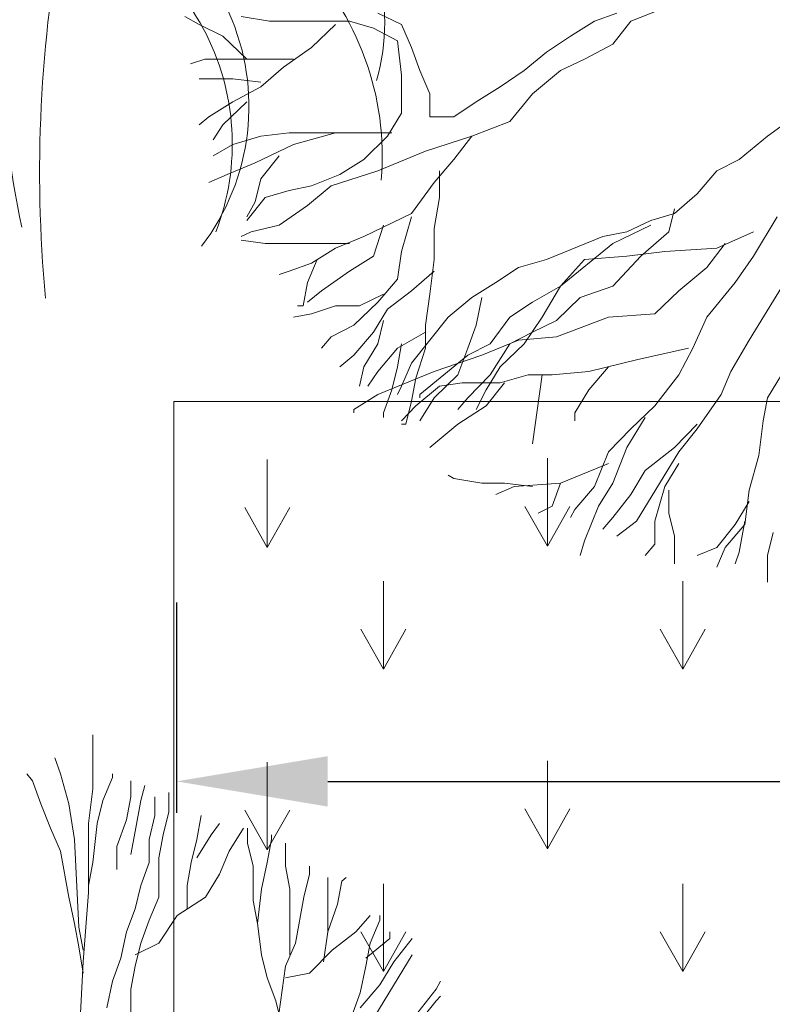
# Model space of a CAD drawing. Units: millimetres. Extents: x 595116 to 630915, y 909473 to 920225.
# Tile 48 of 134: x 629529 to 629559, y 919242 to 919281. Entities that reach past the tile are written whole.
import ezdxf

# ---------------------------------------------------------------- set-up
doc = ezdxf.new("R2010")
doc.units = ezdxf.units.MM
doc.layers.add('Dimension', color=3, linetype='Continuous', lineweight=18)
doc.layers.add('L-PLNT', color=85, linetype='Continuous', lineweight=13)
doc.styles.get("Standard").update_dxf_attribs({"font": 'arial.ttf'})
doc.dimstyles.new('ISO-25', dxfattribs={"dimtxt": 9, "dimasz": 6, "dimexe": 1.25, "dimexo": 0.625, "dimtad": 1, "dimlunit": 4, "dimtxsty": 'Standard', "dimcen": 2.5, "dimadec": 0, "dimazin": 0, "dimtfac": 1, "dimtmove": 0, "dimatfit": 3, "dimfxl": 1, "dimarcsym": 0})

# ---------------------------------------------------------------- blocks, each defined once
blk = doc.blocks.new('tree')
for centre, radius, start, end in [((629595.141, 919296.95), 5.184, 352.032, 57.0714), ((629569.835, 919289.496), 31.168, 13.149, 20.5076), ((629604.232, 919296.737), 3.791, 61.1347, 193.108), ((629594.259, 919292.132), 6.965, 7.4001, 94.0059), ((629589.446, 919288.922), 12.167, 24.2477, 54.3726), ((629605.429, 919293.205), 4.185, 348.9977, 176.315), ((629605.915, 919293.144), 3.963, 69.3845, 175.231), ((629595.377, 919292.044), 4.722, 54.2484, 144.2167), ((629594.88, 919291.171), 5.506, 43.8672, 89.4805), ((629597.025, 919289.989), 5.01, 36.0581, 170.6542), ((629596.464, 919289.874), 4.4, 52.9074, 159.3471), ((629603.809, 919290.469), 3.92, 343.886, 112.2662), ((629598.153, 919288.998), 5.103, 105.3576, 208.8973), ((629597.068, 919289.758), 3.768, 80.4816, 161.0664), ((629601.247, 919287.941), 5.545, 101.0419, 191.8692), ((629614.329, 919289.554), 13.748, 164.5925, 192.323), ((629600.849, 919288.894), 4.324, 322.5461, 85.805), ((629602.329, 919287.957), 5.355, 355.2141, 94.8217), ((629602.391, 919286.088), 6.769, 99.681, 184.5451), ((629600.275, 919288.191), 4.585, 338.7925, 77.6921), ((629626.813, 919287.645), 25.579, 169.0753, 185.2889)]:
    blk.add_arc(centre, radius, start, end)
blk = doc.blocks.new('A$C143125F4')
for p, q in [((2.883, 4.8338), (2.883, 5.0443)), ((2.7571, 4.892), (2.7353, 4.9547)), ((2.6477, 4.8651), (2.6259, 4.892)), ((2.6806, 4.7755), (2.6477, 4.8651)), ((2.79, 4.7755), (2.7571, 4.892)), ((2.9213, 4.789), (2.9596, 4.8786)), ((2.9596, 4.8786), (2.9596, 4.892)), ((3.0307, 4.8024), (3.0307, 4.8651)), ((2.8666, 4.6994), (2.883, 4.8338)), ((3.069, 4.789), (3.0854, 4.8472)), ((2.8994, 4.6994), (2.9213, 4.789)), ((3.0143, 4.7128), (3.0307, 4.8024)), ((3.0471, 4.668), (3.069, 4.789)), ((3.1237, 4.7307), (3.1237, 4.8024)), ((3.1784, 4.7442), (3.1784, 4.8203)), ((2.7189, 4.6814), (2.6806, 4.7755)), ((2.8119, 4.6367), (2.79, 4.7755)), ((2.976, 4.6098), (3.0143, 4.7128)), ((3.1018, 4.6367), (3.1237, 4.7307)), ((3.1565, 4.6546), (3.1784, 4.7442)), ((3.2878, 4.6367), (3.3042, 4.7307)), ((2.7571, 4.5919), (2.7189, 4.6814)), ((2.8666, 4.4306), (2.8666, 4.6994)), ((2.883, 4.5471), (2.8994, 4.6994)), ((3.3425, 4.6546), (3.3753, 4.6994)), ((3.4136, 4.5919), (3.4683, 4.6814)), ((3.4847, 4.6232), (3.4847, 4.6814)), ((2.8283, 4.2962), (2.8119, 4.6367)), ((3.0307, 4.5784), (3.0471, 4.668)), ((3.1018, 4.5471), (3.1018, 4.6367)), ((3.1401, 4.565), (3.1565, 4.6546)), ((3.2659, 4.5471), (3.2878, 4.6367)), ((3.2878, 4.565), (3.3425, 4.6546)), ((3.5613, 4.5471), (3.5777, 4.6367)), ((3.5777, 4.6367), (3.5777, 4.6546)), ((2.976, 4.5202), (2.976, 4.6098)), ((3.5066, 4.5336), (3.4847, 4.6232)), ((3.6324, 4.5336), (3.6324, 4.6232)), ((2.79, 4.4127), (2.7571, 4.5919)), ((3.1401, 4.4127), (3.1401, 4.565)), ((3.3753, 4.5023), (3.4136, 4.5919)), ((2.8666, 4.4575), (2.883, 4.5471)), ((3.069, 4.4575), (3.1018, 4.5471)), ((3.2495, 4.4575), (3.2659, 4.5471)), ((3.5066, 4.3992), (3.5066, 4.5336)), ((3.5394, 4.444), (3.5613, 4.5471)), ((3.6488, 4.444), (3.6324, 4.5336)), ((3.7254, 4.5023), (3.7254, 4.5336)), ((3.3206, 4.4127), (3.3753, 4.5023)), ((3.7035, 4.4127), (3.7254, 4.5023)), ((3.7965, 4.2783), (3.7965, 4.4888)), ((3.8512, 4.4754), (3.8677, 4.4888)), ((3.0471, 4.3679), (3.069, 4.4575)), ((3.2495, 4.3679), (3.2495, 4.4575)), ((3.523, 4.3096), (3.5394, 4.444)), ((3.6488, 4.1887), (3.6488, 4.444)), ((3.8348, 4.3858), (3.8512, 4.4754)), ((2.8119, 4.3096), (2.79, 4.4127)), ((2.8447, 4.1618), (2.8666, 4.4306)), ((3.1018, 4.3231), (3.1401, 4.4127)), ((3.2112, 4.341), (3.3206, 4.4127)), ((3.6707, 4.2335), (3.7035, 4.4127)), ((3.0143, 4.2783), (3.0471, 4.3679)), ((3.523, 4.3096), (3.5066, 4.3992)), ((3.7965, 4.2783), (3.8348, 4.3858)), ((3.1401, 4.2335), (3.2112, 4.341)), ((3.906, 4.2783), (3.9607, 4.341)), ((3.999, 4.3231), (3.999, 4.341)), ((2.8283, 4.22), (2.8119, 4.3096)), ((2.8447, 4.2066), (2.8283, 4.2962)), ((3.069, 4.2335), (3.1018, 4.3231)), ((3.5394, 4.1887), (3.523, 4.3096)), ((3.9607, 4.2335), (3.999, 4.3231)), ((2.9924, 4.1752), (3.0143, 4.2783)), ((3.7801, 4.1618), (3.7965, 4.2783)), ((3.813, 4.2066), (3.906, 4.2783)), ((3.9442, 4.1752), (4.0372, 4.2514)), ((4.0372, 4.2514), (4.0372, 4.2783)), ((4.1248, 4.2514), (4.0537, 4.1618)), ((2.8447, 4.117), (2.8283, 4.22)), ((3.0471, 4.1887), (3.1401, 4.2335)), ((3.0471, 4.1439), (3.069, 4.2335)), ((3.6324, 4.1439), (3.6707, 4.2335)), ((3.9442, 4.1439), (3.9607, 4.2335)), ((2.9596, 4.0856), (2.9924, 4.1752)), ((3.5613, 4.0991), (3.5394, 4.1887)), ((3.7254, 4.117), (3.813, 4.2066)), ((3.9607, 3.9199), (4.1248, 4.1887)), ((2.8283, 3.8303), (2.8447, 4.1618)), ((3.0307, 4.0543), (3.0471, 4.1439)), ((3.5941, 3.8751), (3.6324, 4.1439)), ((3.9224, 4.0408), (3.9442, 4.1439)), ((4.0537, 4.1618), (3.999, 4.0722)), ((3.5941, 4.0095), (3.5613, 4.0991)), ((3.6324, 4.0991), (3.7254, 4.117)), ((2.9377, 3.9826), (2.9596, 4.0856)), ((3.999, 4.0722), (3.9224, 3.9826)), ((4.2178, 4.0543), (4.2342, 4.0856)), ((3.0307, 3.9647), (3.0307, 4.0543)), ((3.8895, 3.9512), (3.9224, 4.0408)), ((4.1467, 3.9647), (4.2178, 4.0543)), ((4.2178, 4.0095), (4.2342, 4.0274)), ((3.616, 3.9199), (3.5941, 4.0095)), ((4.1467, 3.9199), (4.2178, 4.0095)), ((0.7823, 2.231), (0.8753, 2.1862)), ((1.6247, 2.1996), (1.7123, 2.231)), ((1.8819, 2.2444), (1.767, 2.1996)), ((0.0875, 2.1862), (0.0328, 2.2175)), ((0.1805, 2.1414), (0.0875, 2.1862)), ((0.3611, 2.1996), (0.2516, 2.2175)), ((0.6729, 2.1996), (0.3611, 2.1996)), ((0.6182, 2.1862), (0.5252, 2.0966)), ((0.7659, 2.1727), (0.6729, 2.1996)), ((0.8753, 2.1862), (0.9136, 2.0966)), ((1.5317, 2.1414), (1.6247, 2.1996)), ((1.767, 2.1996), (1.6959, 2.11)), ((0.8589, 2.1235), (0.7659, 2.1727)), ((0.2735, 2.0518), (0.1805, 2.1414)), ((0.8753, 1.9891), (0.8589, 2.1235)), ((1.4387, 2.0787), (1.5317, 2.1414)), ((1.6959, 2.11), (1.5865, 2.0518)), ((0.5252, 2.0966), (0.4158, 2.0204)), ((0.9136, 2.0966), (0.9464, 2.007)), ((1.3512, 2.007), (1.4387, 2.0787)), ((0.1094, 2.0518), (0.0547, 2.0339)), ((0.4541, 2.0518), (0.1094, 2.0518)), ((1.5865, 2.0518), (1.4935, 2.007)), ((0.4158, 2.0204), (0.3282, 1.9443)), ((0.9464, 2.007), (0.9847, 1.9174)), ((1.2582, 1.9443), (1.3512, 2.007)), ((1.4935, 2.007), (1.384, 1.9174)), ((0.2188, 1.9756), (0.0875, 1.9756)), ((0.3282, 1.9622), (0.2188, 1.9756)), ((0.8753, 1.8412), (0.8753, 1.9891)), ((0.3282, 1.9443), (0.2188, 1.886)), ((0.9847, 1.9174), (0.9847, 1.8278)), ((1.1652, 1.886), (1.2582, 1.9443)), ((1.384, 1.9174), (1.2965, 1.8099)), ((0.2188, 1.886), (0.1258, 1.8278)), ((0.2735, 1.886), (0.1805, 1.7964)), ((1.0777, 1.8278), (1.1652, 1.886)), ((2.5, 1.8995), (2.2976, 1.7516)), ((0.8206, 1.7516), (0.8753, 1.8412)), ((0.1258, 1.8278), (0.0875, 1.7964)), ((0.9847, 1.8278), (1.0777, 1.8278)), ((1.2965, 1.8099), (1.1488, 1.7516)), ((0.1805, 1.7964), (0.1422, 1.7382)), ((0.4376, 1.7651), (0.3282, 1.7516)), ((0.837, 1.7651), (0.4376, 1.7651)), ((0.6182, 1.7651), (0.4541, 1.7203)), ((0.3282, 1.7516), (0.2188, 1.7203)), ((0.7276, 1.662), (0.8206, 1.7516)), ((1.1488, 1.7516), (0.9683, 1.6934)), ((1.1488, 1.7516), (1.0777, 1.662)), ((2.2976, 1.7516), (2.1882, 1.662)), ((0.2188, 1.7203), (0.1422, 1.6755)), ((0.4541, 1.7203), (0.3063, 1.6486)), ((0.9683, 1.6934), (0.7823, 1.6172)), ((0.3063, 1.6486), (0.1969, 1.6038)), ((0.3993, 1.6755), (0.3282, 1.5859)), ((0.6346, 1.6038), (0.7276, 1.662)), ((1.0777, 1.662), (1.0011, 1.5724)), ((2.1882, 1.662), (2.1007, 1.6172)), ((0.7823, 1.6172), (0.6018, 1.559)), ((1.023, 1.6172), (1.023, 1.5142)), ((2.1007, 1.6172), (2.0241, 1.5276)), ((0.1969, 1.6038), (0.1258, 1.5724)), ((0.3282, 1.5859), (0.3063, 1.4963)), ((0.5252, 1.559), (0.6346, 1.6038)), ((1.0011, 1.5724), (0.9136, 1.4515)), ((0.3446, 1.5142), (0.4376, 1.5411)), ((0.4376, 1.5411), (0.5252, 1.559)), ((0.6018, 1.559), (0.5088, 1.4828)), ((0.2735, 1.4246), (0.3446, 1.5142)), ((0.3063, 1.4963), (0.2735, 1.438)), ((1.023, 1.5142), (1.0011, 1.3932)), ((2.0241, 1.5276), (1.9366, 1.4515)), ((0.5088, 1.4828), (0.3993, 1.4067)), ((1.9366, 1.4694), (1.9147, 1.3798)), ((0.9136, 1.4515), (0.7276, 1.3619)), ((0.9136, 1.438), (0.8753, 1.3036)), ((1.8436, 1.4246), (1.7506, 1.3798)), ((1.9366, 1.4515), (1.8436, 1.4246)), ((2.3359, 1.438), (2.2429, 1.2857)), ((0.2899, 1.3798), (0.2516, 1.3619)), ((0.3993, 1.4067), (0.2899, 1.3798)), ((0.8042, 1.4067), (0.7659, 1.2857)), ((1.0011, 1.3932), (1.0011, 1.2723)), ((1.7506, 1.3798), (1.6576, 1.3619)), ((1.8436, 1.4067), (1.6959, 1.335)), ((1.9147, 1.3798), (1.8053, 1.2857)), ((2.2429, 1.3798), (2.1007, 1.3171)), ((0.3446, 1.335), (0.2516, 1.3484)), ((0.7276, 1.3619), (0.6182, 1.3171)), ((1.6576, 1.3619), (1.4387, 1.2723)), ((0.6729, 1.335), (0.3446, 1.335)), ((0.6182, 1.3171), (0.5252, 1.2588)), ((0.8753, 1.3036), (0.8589, 1.1961)), ((1.6959, 1.335), (1.4935, 1.1692)), ((1.8983, 1.3036), (1.7506, 1.2857)), ((2.1007, 1.3171), (1.8983, 1.3036)), ((2.1335, 1.335), (2.0624, 1.2409)), ((0.5471, 1.2723), (0.5088, 1.1827)), ((0.7659, 1.2857), (0.6729, 1.2275)), ((1.0011, 1.2723), (0.9847, 1.1379)), ((1.4387, 1.2723), (1.3293, 1.2409)), ((1.5865, 1.2723), (1.4935, 1.1692)), ((1.7506, 1.2857), (1.5865, 1.2723)), ((1.8053, 1.2857), (1.6959, 1.1692)), ((2.2429, 1.2857), (2.1718, 1.1827)), ((0.4376, 1.2275), (0.3993, 1.214)), ((0.5252, 1.2588), (0.4376, 1.2275)), ((0.6729, 1.2275), (0.5635, 1.1513)), ((1.0011, 1.2275), (0.9136, 1.1513)), ((1.3293, 1.2409), (1.2418, 1.1827)), ((2.0624, 1.2409), (1.953, 1.1513)), ((2.3906, 1.2275), (2.2265, 0.9587)), ((0.8589, 1.1961), (0.7823, 1.1065)), ((0.5088, 1.1827), (0.4923, 1.0931)), ((0.5635, 1.1513), (0.5088, 1.1065)), ((0.9136, 1.1513), (0.8206, 1.0796)), ((1.2418, 1.1827), (1.1488, 1.1244)), ((1.4935, 1.1692), (1.384, 1.1065)), ((1.4935, 1.1692), (1.4223, 1.0483)), ((1.6959, 1.1692), (1.57, 1.1244)), ((1.953, 1.1513), (1.86, 1.0617)), ((2.1718, 1.1827), (2.0624, 1.0483)), ((0.8042, 1.1379), (0.7112, 1.0931)), ((0.9847, 1.1379), (0.9683, 1.0169)), ((1.1488, 1.1244), (1.0558, 1.0483)), ((1.1871, 1.1244), (1.1652, 1.0169)), ((1.57, 1.1244), (1.477, 1.0348)), ((0.4923, 1.0931), (0.4705, 1.0931)), ((0.6182, 1.0931), (0.5252, 1.0617)), ((0.7112, 1.0931), (0.6182, 1.0931)), ((0.7823, 1.1065), (0.6893, 1.0169)), ((0.8206, 1.0796), (0.7659, 0.99)), ((1.384, 1.1065), (1.2965, 1.0483)), ((0.5252, 1.0617), (0.4541, 1.0483)), ((0.8042, 1.0348), (0.7823, 0.9452)), ((1.0558, 1.0483), (0.9136, 0.8691)), ((1.2965, 1.0483), (1.2199, 0.9452)), ((1.4223, 1.0483), (1.3512, 0.9452)), ((1.477, 1.0348), (1.384, 0.99)), ((1.6795, 1.0483), (1.477, 0.9721)), ((1.86, 1.0617), (1.6795, 1.0483)), ((2.0624, 1.0483), (2.0077, 0.9273)), ((0.6893, 1.0169), (0.6018, 0.9721)), ((0.9683, 1.0169), (0.9683, 0.9273)), ((1.1652, 1.0169), (1.1324, 0.9273)), ((0.6018, 0.9721), (0.5635, 0.9273)), ((0.7659, 0.99), (0.6893, 0.9005)), ((0.9683, 0.99), (0.8589, 0.9273)), ((1.3293, 0.9587), (1.1871, 0.9005)), ((1.384, 0.99), (1.2965, 0.9452)), ((1.477, 0.9721), (1.3293, 0.9587)), ((2.2265, 0.9587), (2.1554, 0.8377)), ((0.7823, 0.9452), (0.7276, 0.8557)), ((0.8589, 0.9273), (0.7823, 0.8377)), ((0.8753, 0.9452), (0.8589, 0.8557)), ((0.9683, 0.9273), (0.93, 0.8109)), ((1.1324, 0.9273), (1.0941, 0.8243)), ((1.2199, 0.9452), (1.1324, 0.9005)), ((1.2965, 0.9452), (1.2199, 0.8243)), ((1.3512, 0.9452), (1.2582, 0.8557)), ((1.9913, 0.9273), (1.7889, 0.8825)), ((2.0077, 0.9273), (1.953, 0.8243)), ((0.6893, 0.9005), (0.6346, 0.8557)), ((1.1324, 0.9005), (0.9464, 0.7481)), ((1.1871, 0.9005), (1.0011, 0.8377)), ((1.7889, 0.8825), (1.6029, 0.8377)), ((0.7276, 0.8557), (0.7112, 0.7795)), ((0.8589, 0.8557), (0.837, 0.7661)), ((0.9136, 0.8691), (0.8753, 0.7795)), ((1.2582, 0.8557), (1.2035, 0.7661)), ((1.6795, 0.8557), (1.6029, 0.7661)), ((0.7823, 0.8377), (0.744, 0.7795)), ((1.0011, 0.8377), (0.7823, 0.7481)), ((0.93, 0.8109), (0.9136, 0.7213)), ((1.0941, 0.8243), (1.0011, 0.7347)), ((1.2199, 0.8243), (1.1324, 0.7347)), ((1.3676, 0.8243), (1.2582, 0.7929)), ((1.4606, 0.8243), (1.3676, 0.8243)), ((1.4223, 0.8243), (1.384, 0.5555)), ((1.6029, 0.8377), (1.4606, 0.8243)), ((1.953, 0.8243), (1.86, 0.7033)), ((2.1554, 0.8377), (2.1171, 0.7481)), ((2.3523, 0.8243), (2.2976, 0.7347)), ((0.837, 0.7661), (0.8042, 0.6765)), ((0.8753, 0.7795), (0.8589, 0.7481)), ((1.023, 0.7795), (0.93, 0.7033)), ((1.1105, 0.7929), (1.023, 0.7795)), ((1.2582, 0.7929), (1.1105, 0.7929)), ((1.2035, 0.7661), (1.1652, 0.6899)), ((1.2746, 0.7929), (1.2035, 0.7033)), ((1.6029, 0.7661), (1.5482, 0.6765)), ((0.7823, 0.7481), (0.6893, 0.6899)), ((0.9464, 0.7481), (0.9464, 0.7347)), ((1.0011, 0.7347), (0.9464, 0.6451)), ((1.1324, 0.7347), (1.0941, 0.6899)), ((2.1171, 0.7481), (2.0241, 0.6137)), ((2.2976, 0.7347), (2.2812, 0.6451)), ((0.6893, 0.6899), (0.6893, 0.6765)), ((0.93, 0.7033), (0.8753, 0.6451)), ((0.9136, 0.7213), (0.8917, 0.6317)), ((1.2035, 0.7033), (1.0941, 0.6317)), ((1.86, 0.7033), (1.767, 0.6137)), ((0.8042, 0.6765), (0.8042, 0.6585)), ((1.5482, 0.6765), (1.5482, 0.6451)), ((1.8217, 0.6585), (1.7506, 0.5421)), ((0.8917, 0.6317), (0.8753, 0.6317)), ((1.0941, 0.6317), (0.9847, 0.5421)), ((1.767, 0.6137), (1.6795, 0.5241)), ((2.0241, 0.6317), (1.9366, 0.5421)), ((2.0241, 0.6137), (1.953, 0.5241)), ((2.2812, 0.6451), (2.2648, 0.5107)), ((1.7506, 0.5421), (1.6959, 0.4032)), ((1.9366, 0.5421), (1.8217, 0.4525)), ((1.6795, 0.5241), (1.6247, 0.3897)), ((1.953, 0.5241), (1.7889, 0.2554)), ((2.2648, 0.5107), (2.2265, 0.3763)), ((1.6795, 0.4793), (1.4935, 0.4032)), ((1.953, 0.4793), (1.8983, 0.3897)), ((1.0777, 0.4211), (1.0558, 0.4345)), ((1.8217, 0.4525), (1.767, 0.3584)), ((1.1871, 0.4032), (1.0777, 0.4211)), ((1.2746, 0.4032), (1.1871, 0.4032)), ((1.3129, 0.3897), (1.2418, 0.3584)), ((1.384, 0.3897), (1.2746, 0.4032)), ((1.4935, 0.4032), (1.3129, 0.3897)), ((1.4935, 0.4032), (1.4606, 0.3136)), ((1.6247, 0.3897), (1.5482, 0.3002)), ((1.6959, 0.4032), (1.6412, 0.3136)), ((1.8983, 0.3897), (1.86, 0.2554)), ((1.767, 0.3584), (1.6959, 0.2688)), ((1.9147, 0.3763), (1.9147, 0.2867)), ((2.2265, 0.3763), (2.2101, 0.2419)), ((1.4606, 0.3136), (1.4059, 0.2867)), ((1.6412, 0.3136), (1.5865, 0.1792)), ((2.2265, 0.3315), (2.1718, 0.2419)), ((1.5482, 0.3002), (1.5317, 0.2688)), ((1.6959, 0.2688), (1.6576, 0.224)), ((1.9147, 0.2867), (1.9366, 0.1971)), ((1.7889, 0.2554), (1.7123, 0.1971)), ((1.86, 0.2554), (1.86, 0.1658)), ((2.1718, 0.2419), (2.1007, 0.1523)), ((2.2101, 0.2419), (2.1335, 0.1523)), ((2.2101, 0.2554), (2.1882, 0.1344)), ((1.9366, 0.1971), (1.9366, 0.0896)), ((2.2976, 0.121), (2.3195, 0.2106)), ((1.5865, 0.1792), (1.57, 0.121)), ((1.86, 0.1658), (1.8217, 0.121)), ((2.1007, 0.1523), (2.0241, 0.121)), ((2.1335, 0.1523), (2.1007, 0.0762)), ((2.1882, 0.1344), (2.1718, 0.0896)), ((2.2976, 0.0179), (2.2976, 0.121))]:
    blk.add_line(p, q)
blk = doc.blocks.new('LAWN-GRASS-TUFT')
blk.add_line((0.892, 3.485), (0.892, 0))
blk.add_lwpolyline([(0, 1.577), (0.892, 0), (1.785, 1.577)])
blk = doc.blocks.new('*D211')
at = {"layer": 'Defpoints', "color": 0, "transparency": 16777216}
for p in [(629535.386, 919258.662), (629586.227, 919258.662), (629586.227, 919250.943)]:
    blk.add_point(p, dxfattribs=at)
at = {"layer": 'Dimension', "color": 0, "lineweight": -2, "transparency": 16777216}
for p, q in [((629535.386, 919258.037), (629535.386, 919249.693)), ((629586.227, 919258.037), (629586.227, 919249.693)), ((629541.386, 919250.943), (629580.227, 919250.943)), ((629586.227, 919250.943), (629648.699, 919250.943))]:
    blk.add_line(p, q, dxfattribs=at)
at = {"layer": 'Dimension', "color": 0, "transparency": 16777216}
for points in [[(629541.386, 919251.943), (629541.386, 919249.943), (629535.386, 919250.943)], [(629580.227, 919251.943), (629580.227, 919249.943), (629586.227, 919250.943)]]:
    blk.add_solid(points, dxfattribs=at)
at = {"layer": 'Dimension', "color": 0, "transparency": 16777216, "insert": (629620.463, 919256.167), "char_height": 9, "attachment_point": 5}
blk.add_mtext('4\'-3" TYP.', dxfattribs=at)
blk = doc.blocks.new('*D216')
at = {"layer": 'Defpoints', "color": 0, "transparency": 16777216}
for p in [(629743.541, 919411.928), (629505.041, 919411.828), (629743.541, 918832.378)]:
    blk.add_point(p, dxfattribs=at)
at = {"layer": 'Dimension', "color": 0, "lineweight": -2, "transparency": 16777216}
for p, q in [((629505.041, 919411.203), (629505.041, 918831.128)), ((629743.541, 919411.303), (629743.541, 918831.128)), ((629511.041, 918832.378), (629737.541, 918832.378))]:
    blk.add_line(p, q, dxfattribs=at)
at = {"layer": 'Dimension', "color": 0, "transparency": 16777216}
for points in [[(629511.041, 918833.378), (629511.041, 918831.378), (629505.041, 918832.378)], [(629737.541, 918833.378), (629737.541, 918831.378), (629743.541, 918832.378)]]:
    blk.add_solid(points, dxfattribs=at)
at = {"layer": 'Dimension', "color": 0, "transparency": 16777216, "insert": (629624.291, 918837.656), "char_height": 9, "attachment_point": 5}
blk.add_mtext('19\'-10 1/2"', dxfattribs=at)

msp = doc.modelspace()

# ---------------------------------------------------------------- linework, layer by layer
at = {"layer": 'L-PLNT'}
for p, q in [((629800.951, 919266.009), (629535.274, 919266.009)), ((629535.274, 919266.009), (629535.274, 919184.917))]:
    msp.add_line(p, q, dxfattribs=at)

# ---------------------------------------------------------------- block references
for name, p, xscale, yscale, zscale in [('A$C143125F4', (629535.386, 919258.662), 10.20167662382051, 10.20167662382051, 10.20167662382051), ('tree', (-697473.9, -1018297.752), 2.107689410566463, 2.107689410566463, 2.107689410566463), ('A$C143125F4', (629502.654, 919201.332), 10.20167662382051, 10.20167662382051, 10.20167662382051)]:
    msp.add_blockref(name, p, dxfattribs=dict(at, xscale=xscale, yscale=yscale, zscale=zscale))
for p in [(629538.093, 919260.225), (629549.207, 919260.275), (629542.7, 919255.397), (629554.573, 919255.397), (629538.093, 919248.223), (629549.207, 919248.272), (629542.7, 919243.395), (629554.573, 919243.395)]:
    msp.add_blockref('LAWN-GRASS-TUFT', p, dxfattribs=at)

# ---------------------------------------------------------------- dimensions: what is measured, and where the dimension line sits
at = {"layer": 'Dimension'}
dim = msp.add_linear_dim(base=(629743.541, 918832.378), p1=(629505.041, 919411.828), p2=(629743.541, 919411.928), dimstyle='ISO-25', override={"dimdec": 1, "dimlfac": 1, "dimrnd": 0, "dimzin": 1, "dimdsep": 46, "dimlunit": 4, "dimfrac": 2}, dxfattribs=at)
dim.commit()
dim.dimension.update_dxf_attribs({"geometry": '*D216', "text_midpoint": (629624.291, 918837.656)})
dim = msp.add_linear_dim(base=(629586.227, 919250.943), p1=(629535.386, 919258.662), p2=(629586.227, 919258.662), text='<> TYP.', dimstyle='ISO-25', override={"dimdec": 1, "dimlfac": 1, "dimrnd": 0, "dimzin": 1, "dimdsep": 46, "dimlunit": 4, "dimfrac": 2}, dxfattribs=at)
dim.commit()
dim.dimension.update_dxf_attribs({"geometry": '*D211', "text_midpoint": (629620.463, 919256.167)})

doc.saveas('drawing.dxf')
